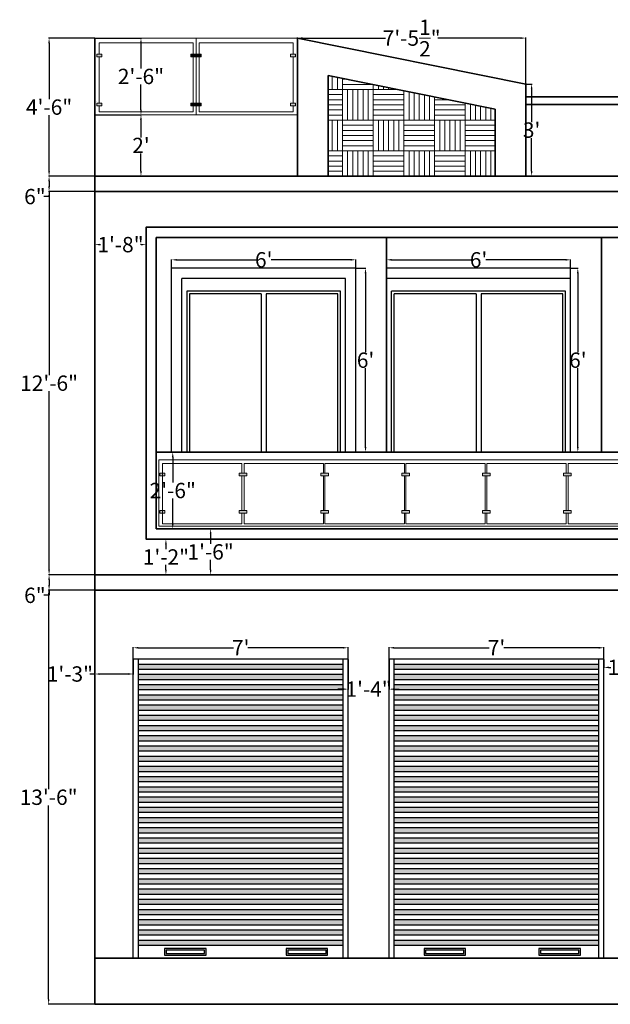
# Model space of a CAD drawing. Units: inches. Extents: x 786 to 1239, y 110 to 563.
# Tile 1 of 3: x 786 to 1017, y 110 to 495. Entities that reach past the tile are written whole.
import ezdxf

# ---------------------------------------------------------------- set-up
doc = ezdxf.new("R2010")
doc.units = ezdxf.units.IN
doc.header["$MEASUREMENT"] = 0
for name, color, linetype, lineweight in [('A-ANNO-DIMS', 2, 'Continuous', 18), ('A-DOOR', 4, 'Continuous', 25), ('A-ELEV', 7, 'Continuous', 35), ('A-ELEV-PATT', 8, 'Continuous', 13), ('A-ELEV-RAIL', 3, 'Continuous', 18), ('A-GLAZ', 4, 'Continuous', 25)]:
    doc.layers.add(name, color=color, linetype=linetype, lineweight=lineweight)
doc.styles.get("Standard").update_dxf_attribs({"font": 'arial.ttf'})
doc.dimstyles.get("Standard").update_dxf_attribs({"dimtxt": 6, "dimasz": 2, "dimexe": 0.18, "dimexo": 0.0625, "dimgap": 0.09, "dimtad": 0, "dimtih": 1, "dimtoh": 1, "dimdec": 1, "dimzin": 0, "dimdsep": 46, "dimlunit": 4, "dimtxsty": 'Standard', "dimcen": 0.09, "dimadec": 0, "dimazin": 0, "dimtfac": 1, "dimtdec": 1, "dimtofl": 0, "dimtmove": 0, "dimatfit": 3, "dimfxl": 1, "dimtolj": 1, "dimtzin": 0, "dimarcsym": 0})

# ---------------------------------------------------------------- blocks, each defined once
blk = doc.blocks.new('*D7')
at = {"layer": 'A-ANNO-DIMS', "color": 0, "lineweight": -2, "transparency": 16777216}
for p, q in [((1035.19, 272.05), (1035.19, 241.73)), ((1014.19, 245.05), (1014.19, 241.73)), ((1016.19, 241.91), (1016.91, 241.91)), ((1033.19, 241.91), (1032.48, 241.91))]:
    blk.add_line(p, q, dxfattribs=at)
at = {"layer": 'A-ANNO-DIMS', "color": 0, "transparency": 16777216}
for points in [[(1016.19, 242.24), (1016.19, 241.58), (1014.19, 241.91)], [(1033.19, 242.24), (1033.19, 241.58), (1035.19, 241.91)]]:
    blk.add_solid(points, dxfattribs=at)
at = {"layer": 'Defpoints', "color": 0, "transparency": 16777216}
for p in [(1035.19, 272.11), (1014.19, 245.11), (1035.19, 241.91)]:
    blk.add_point(p, dxfattribs=at)
at = {"layer": 'A-ANNO-DIMS', "color": 0, "transparency": 16777216, "insert": (1024.69, 241.91), "char_height": 6, "attachment_point": 5}
blk.add_mtext('\\A1;1\'-9"', dxfattribs=at)
blk = doc.blocks.new('*D8')
at = {"layer": 'A-ANNO-DIMS', "color": 0, "lineweight": -2, "transparency": 16777216}
for p, q in [((815.19, 272.05), (815.19, 239.15)), ((830.19, 245.05), (830.19, 239.15)), ((815.19, 239.33), (813.19, 239.33)), ((828.19, 239.33), (817.19, 239.33))]:
    blk.add_line(p, q, dxfattribs=at)
at = {"layer": 'A-ANNO-DIMS', "color": 0, "transparency": 16777216}
for points in [[(817.19, 239.66), (817.19, 238.99), (815.19, 239.33)], [(828.19, 239.66), (828.19, 238.99), (830.19, 239.33)]]:
    blk.add_solid(points, dxfattribs=at)
at = {"layer": 'Defpoints', "color": 0, "transparency": 16777216}
for p in [(815.19, 272.11), (830.19, 245.11), (815.19, 239.33)]:
    blk.add_point(p, dxfattribs=at)
at = {"layer": 'A-ANNO-DIMS', "color": 0, "transparency": 16777216, "insert": (805.41, 239.33), "char_height": 6, "attachment_point": 5}
blk.add_mtext('\\A1;1\'-3"', dxfattribs=at)
blk = doc.blocks.new('*D12')
at = {"layer": 'A-ANNO-DIMS', "color": 0, "lineweight": -2, "transparency": 16777216}
for p, q in [((815.19, 428.05), (815.19, 407.13)), ((835.19, 410.05), (835.19, 407.13)), ((817.19, 407.31), (817.41, 407.31)), ((833.19, 407.31), (832.98, 407.31))]:
    blk.add_line(p, q, dxfattribs=at)
at = {"layer": 'A-ANNO-DIMS', "color": 0, "transparency": 16777216}
for points in [[(817.19, 407.64), (817.19, 406.98), (815.19, 407.31)], [(833.19, 407.64), (833.19, 406.98), (835.19, 407.31)]]:
    blk.add_solid(points, dxfattribs=at)
at = {"layer": 'Defpoints', "color": 0, "transparency": 16777216}
for p in [(815.19, 428.11), (835.19, 410.11), (835.19, 407.31)]:
    blk.add_point(p, dxfattribs=at)
at = {"layer": 'A-ANNO-DIMS', "color": 0, "transparency": 16777216, "insert": (825.19, 407.31), "char_height": 6, "attachment_point": 5}
blk.add_mtext('\\A1;1\'-8"', dxfattribs=at)
blk = doc.blocks.new('*D13')
at = {"layer": 'A-ANNO-DIMS', "color": 0, "lineweight": -2, "transparency": 16777216}
for p, q in [((839.26, 326.11), (845.81, 326.11)), ((845.63, 324.11), (845.63, 314.26)), ((845.63, 298.11), (845.63, 307.96)), ((839.26, 296.11), (845.81, 296.11))]:
    blk.add_line(p, q, dxfattribs=at)
at = {"layer": 'A-ANNO-DIMS', "color": 0, "transparency": 16777216}
for points in [[(845.3, 324.11), (845.97, 324.11), (845.63, 326.11)], [(845.3, 298.11), (845.97, 298.11), (845.63, 296.11)]]:
    blk.add_solid(points, dxfattribs=at)
at = {"layer": 'Defpoints', "color": 0, "transparency": 16777216}
for p in [(839.19, 326.11), (839.19, 296.11), (845.63, 296.11)]:
    blk.add_point(p, dxfattribs=at)
at = {"layer": 'A-ANNO-DIMS', "color": 0, "transparency": 16777216, "insert": (845.63, 311.11), "char_height": 6, "attachment_point": 5}
blk.add_mtext('\\A1;2\'-6"', dxfattribs=at)
blk = doc.blocks.new('*D24')
at = {"layer": 'A-ANNO-DIMS', "color": 0, "lineweight": -2, "transparency": 16777216}
for p, q in [((835.26, 292.11), (843.14, 292.11)), ((842.96, 290.11), (842.96, 288.21)), ((842.96, 280.11), (842.96, 282.01)), ((815.26, 278.11), (843.14, 278.11))]:
    blk.add_line(p, q, dxfattribs=at)
at = {"layer": 'A-ANNO-DIMS', "color": 0, "transparency": 16777216}
for points in [[(842.63, 290.11), (843.29, 290.11), (842.96, 292.11)], [(842.63, 280.11), (843.29, 280.11), (842.96, 278.11)]]:
    blk.add_solid(points, dxfattribs=at)
at = {"layer": 'Defpoints', "color": 0, "transparency": 16777216}
for p in [(835.19, 292.11), (842.96, 292.11), (815.19, 278.11)]:
    blk.add_point(p, dxfattribs=at)
at = {"layer": 'A-ANNO-DIMS', "color": 0, "transparency": 16777216, "insert": (842.96, 285.11), "char_height": 6, "attachment_point": 5}
blk.add_mtext('\\A1;1\'-2"', dxfattribs=at)
blk = doc.blocks.new('*D25')
at = {"layer": 'A-ANNO-DIMS', "color": 0, "lineweight": -2, "transparency": 16777216}
for p, q in [((839.26, 296.11), (860.61, 296.11)), ((860.43, 294.11), (860.43, 290.26)), ((860.43, 280.11), (860.43, 283.96)), ((815.26, 278.11), (860.61, 278.11))]:
    blk.add_line(p, q, dxfattribs=at)
at = {"layer": 'A-ANNO-DIMS', "color": 0, "transparency": 16777216}
for points in [[(860.1, 294.11), (860.77, 294.11), (860.43, 296.11)], [(860.1, 280.11), (860.77, 280.11), (860.43, 278.11)]]:
    blk.add_solid(points, dxfattribs=at)
at = {"layer": 'Defpoints', "color": 0, "transparency": 16777216}
for p in [(839.19, 296.11), (860.43, 296.11), (815.19, 278.11)]:
    blk.add_point(p, dxfattribs=at)
at = {"layer": 'A-ANNO-DIMS', "color": 0, "transparency": 16777216, "insert": (860.43, 287.11), "char_height": 6, "attachment_point": 5}
blk.add_mtext('\\A1;1\'-6"', dxfattribs=at)
blk = doc.blocks.new('*D26')
at = {"layer": 'A-ANNO-DIMS', "color": 0, "lineweight": -2, "transparency": 16777216}
for p, q in [((894.39, 488.17), (894.39, 488.29)), ((896.39, 488.11), (928.8, 488.11)), ((981.67, 488.11), (949.26, 488.11)), ((983.67, 470.19), (983.67, 488.29))]:
    blk.add_line(p, q, dxfattribs=at)
at = {"layer": 'A-ANNO-DIMS', "color": 0, "transparency": 16777216}
for points in [[(896.39, 488.44), (896.39, 487.78), (894.39, 488.11)], [(981.67, 488.44), (981.67, 487.78), (983.67, 488.11)]]:
    blk.add_solid(points, dxfattribs=at)
at = {"layer": 'Defpoints', "color": 0, "transparency": 16777216}
for p in [(894.39, 488.11), (894.39, 488.11), (983.67, 470.13)]:
    blk.add_point(p, dxfattribs=at)
at = {"layer": 'A-ANNO-DIMS', "color": 0, "transparency": 16777216, "insert": (939.03, 488.11), "char_height": 6, "attachment_point": 5}
blk.add_mtext('\\A1;7\'-5{\\H1x;\\S1/2;}"', dxfattribs=at)
blk = doc.blocks.new('*D27')
at = {"layer": 'A-ANNO-DIMS', "color": 0, "lineweight": -2, "transparency": 16777216}
for p, q in [((983.73, 470.13), (986.11, 470.13)), ((985.93, 468.13), (985.93, 455.27)), ((985.93, 436.11), (985.93, 448.96)), ((983.73, 434.11), (986.11, 434.11))]:
    blk.add_line(p, q, dxfattribs=at)
at = {"layer": 'A-ANNO-DIMS', "color": 0, "transparency": 16777216}
for points in [[(985.6, 468.13), (986.27, 468.13), (985.93, 470.13)], [(985.6, 436.11), (986.27, 436.11), (985.93, 434.11)]]:
    blk.add_solid(points, dxfattribs=at)
at = {"layer": 'Defpoints', "color": 0, "transparency": 16777216}
for p in [(983.67, 470.13), (985.93, 470.13), (983.67, 434.11)]:
    blk.add_point(p, dxfattribs=at)
at = {"layer": 'A-ANNO-DIMS', "color": 0, "transparency": 16777216, "insert": (985.93, 452.12), "char_height": 6, "attachment_point": 5}
blk.add_mtext("\\A1;3'", dxfattribs=at)
blk = doc.blocks.new('*D28')
at = {"layer": 'A-ANNO-DIMS', "color": 0, "lineweight": -2, "transparency": 16777216}
for p, q in [((815.26, 488.11), (833.38, 488.11)), ((833.2, 486.11), (833.2, 476.26)), ((833.2, 460.11), (833.2, 469.96)), ((815.26, 458.11), (833.38, 458.11))]:
    blk.add_line(p, q, dxfattribs=at)
at = {"layer": 'A-ANNO-DIMS', "color": 0, "transparency": 16777216}
for points in [[(832.86, 486.11), (833.53, 486.11), (833.2, 488.11)], [(832.86, 460.11), (833.53, 460.11), (833.2, 458.11)]]:
    blk.add_solid(points, dxfattribs=at)
at = {"layer": 'Defpoints', "color": 0, "transparency": 16777216}
for p in [(815.19, 488.11), (815.19, 458.11), (833.2, 458.11)]:
    blk.add_point(p, dxfattribs=at)
at = {"layer": 'A-ANNO-DIMS', "color": 0, "transparency": 16777216, "insert": (833.2, 473.11), "char_height": 6, "attachment_point": 5}
blk.add_mtext('\\A1;2\'-6"', dxfattribs=at)
blk = doc.blocks.new('*D29')
at = {"layer": 'A-ANNO-DIMS', "color": 0, "lineweight": -2, "transparency": 16777216}
for p, q in [((815.26, 458.11), (833.38, 458.11)), ((833.2, 456.11), (833.2, 449.21)), ((833.2, 436.11), (833.2, 443.01)), ((815.26, 434.11), (833.38, 434.11))]:
    blk.add_line(p, q, dxfattribs=at)
at = {"layer": 'A-ANNO-DIMS', "color": 0, "transparency": 16777216}
for points in [[(832.86, 456.11), (833.53, 456.11), (833.2, 458.11)], [(832.86, 436.11), (833.53, 436.11), (833.2, 434.11)]]:
    blk.add_solid(points, dxfattribs=at)
at = {"layer": 'Defpoints', "color": 0, "transparency": 16777216}
for p in [(815.19, 458.11), (815.19, 434.11), (833.2, 434.11)]:
    blk.add_point(p, dxfattribs=at)
at = {"layer": 'A-ANNO-DIMS', "color": 0, "transparency": 16777216, "insert": (833.2, 446.11), "char_height": 6, "attachment_point": 5}
blk.add_mtext("\\A1;2'", dxfattribs=at)
blk = doc.blocks.new('*D30')
at = {"layer": 'A-ANNO-DIMS', "color": 0, "lineweight": -2, "transparency": 16777216}
for p, q in [((830.19, 245.17), (830.19, 249.77)), ((832.19, 249.59), (869.37, 249.59)), ((912.19, 249.59), (875.02, 249.59)), ((914.19, 245.17), (914.19, 249.77))]:
    blk.add_line(p, q, dxfattribs=at)
at = {"layer": 'A-ANNO-DIMS', "color": 0, "transparency": 16777216}
for points in [[(832.19, 249.92), (832.19, 249.26), (830.19, 249.59)], [(912.19, 249.92), (912.19, 249.26), (914.19, 249.59)]]:
    blk.add_solid(points, dxfattribs=at)
at = {"layer": 'Defpoints', "color": 0, "transparency": 16777216}
for p in [(830.19, 249.59), (830.19, 245.11), (914.19, 245.11)]:
    blk.add_point(p, dxfattribs=at)
at = {"layer": 'A-ANNO-DIMS', "color": 0, "transparency": 16777216, "insert": (872.19, 249.59), "char_height": 6, "attachment_point": 5}
blk.add_mtext("\\A1;7'", dxfattribs=at)
blk = doc.blocks.new('*D31')
at = {"layer": 'A-ANNO-DIMS', "color": 0, "lineweight": -2, "transparency": 16777216}
for p, q in [((930.19, 245.17), (930.19, 249.77)), ((932.19, 249.59), (969.37, 249.59)), ((1012.19, 249.59), (975.02, 249.59)), ((1014.19, 245.17), (1014.19, 249.77))]:
    blk.add_line(p, q, dxfattribs=at)
at = {"layer": 'A-ANNO-DIMS', "color": 0, "transparency": 16777216}
for points in [[(932.19, 249.92), (932.19, 249.26), (930.19, 249.59)], [(1012.19, 249.92), (1012.19, 249.26), (1014.19, 249.59)]]:
    blk.add_solid(points, dxfattribs=at)
at = {"layer": 'Defpoints', "color": 0, "transparency": 16777216}
for p in [(930.19, 249.59), (930.19, 245.11), (1014.19, 245.11)]:
    blk.add_point(p, dxfattribs=at)
at = {"layer": 'A-ANNO-DIMS', "color": 0, "transparency": 16777216, "insert": (972.19, 249.59), "char_height": 6, "attachment_point": 5}
blk.add_mtext("\\A1;7'", dxfattribs=at)
blk = doc.blocks.new('*D32')
at = {"layer": 'A-ANNO-DIMS', "color": 0, "lineweight": -2, "transparency": 16777216}
for p, q in [((914.19, 245.05), (914.19, 233.22)), ((930.19, 245.05), (930.19, 233.22)), ((912.19, 233.4), (910.19, 233.4)), ((932.19, 233.4), (934.19, 233.4))]:
    blk.add_line(p, q, dxfattribs=at)
at = {"layer": 'A-ANNO-DIMS', "color": 0, "transparency": 16777216}
for points in [[(912.19, 233.74), (912.19, 233.07), (914.19, 233.4)], [(932.19, 233.74), (932.19, 233.07), (930.19, 233.4)]]:
    blk.add_solid(points, dxfattribs=at)
at = {"layer": 'Defpoints', "color": 0, "transparency": 16777216}
for p in [(914.19, 245.11), (930.19, 245.11), (930.19, 233.4)]:
    blk.add_point(p, dxfattribs=at)
at = {"layer": 'A-ANNO-DIMS', "color": 0, "transparency": 16777216, "insert": (922.19, 233.4), "char_height": 6, "attachment_point": 5}
blk.add_mtext('\\A1;1\'-4"', dxfattribs=at)
blk = doc.blocks.new('*D43')
at = {"layer": 'A-ANNO-DIMS', "color": 0, "lineweight": -2, "transparency": 16777216}
for p, q in [((815.13, 278.11), (797.1, 278.11)), ((797.28, 276.11), (797.28, 274.11)), ((797.28, 270.11), (795.28, 270.11)), ((815.13, 272.11), (797.1, 272.11)), ((797.28, 272.11), (797.28, 270.11))]:
    blk.add_line(p, q, dxfattribs=at)
at = {"layer": 'A-ANNO-DIMS', "color": 0, "transparency": 16777216}
for points in [[(796.95, 276.11), (797.61, 276.11), (797.28, 278.11)], [(796.95, 274.11), (797.61, 274.11), (797.28, 272.11)]]:
    blk.add_solid(points, dxfattribs=at)
at = {"layer": 'Defpoints', "color": 0, "transparency": 16777216}
for p in [(815.19, 278.11), (797.28, 272.11), (815.19, 272.11)]:
    blk.add_point(p, dxfattribs=at)
at = {"layer": 'A-ANNO-DIMS', "color": 0, "transparency": 16777216, "insert": (791.73, 270.11), "char_height": 6, "attachment_point": 5}
blk.add_mtext('\\A1;6"', dxfattribs=at)
blk = doc.blocks.new('*D44')
at = {"layer": 'A-ANNO-DIMS', "color": 0, "lineweight": -2, "transparency": 16777216}
for p, q in [((815.13, 272.11), (796.92, 272.11)), ((797.1, 270.11), (797.1, 194.26)), ((797.1, 112.11), (797.1, 187.95)), ((815.13, 110.11), (796.92, 110.11))]:
    blk.add_line(p, q, dxfattribs=at)
at = {"layer": 'A-ANNO-DIMS', "color": 0, "transparency": 16777216}
for points in [[(796.77, 270.11), (797.43, 270.11), (797.1, 272.11)], [(796.77, 112.11), (797.43, 112.11), (797.1, 110.11)]]:
    blk.add_solid(points, dxfattribs=at)
at = {"layer": 'Defpoints', "color": 0, "transparency": 16777216}
for p in [(815.19, 272.11), (797.1, 110.11), (815.19, 110.11)]:
    blk.add_point(p, dxfattribs=at)
at = {"layer": 'A-ANNO-DIMS', "color": 0, "transparency": 16777216, "insert": (797.1, 191.11), "char_height": 6, "attachment_point": 5}
blk.add_mtext('\\A1;13\'-6"', dxfattribs=at)
blk = doc.blocks.new('*D45')
at = {"layer": 'A-ANNO-DIMS', "color": 0, "lineweight": -2, "transparency": 16777216}
for p, q in [((815.13, 428.11), (797.1, 428.11)), ((797.28, 426.11), (797.28, 356.26)), ((797.28, 280.11), (797.28, 349.96)), ((815.13, 278.11), (797.1, 278.11))]:
    blk.add_line(p, q, dxfattribs=at)
at = {"layer": 'A-ANNO-DIMS', "color": 0, "transparency": 16777216}
for points in [[(796.95, 426.11), (797.61, 426.11), (797.28, 428.11)], [(796.95, 280.11), (797.61, 280.11), (797.28, 278.11)]]:
    blk.add_solid(points, dxfattribs=at)
at = {"layer": 'Defpoints', "color": 0, "transparency": 16777216}
for p in [(797.28, 428.11), (815.19, 428.11), (815.19, 278.11)]:
    blk.add_point(p, dxfattribs=at)
at = {"layer": 'A-ANNO-DIMS', "color": 0, "transparency": 16777216, "insert": (797.28, 353.11), "char_height": 6, "attachment_point": 5}
blk.add_mtext('\\A1;12\'-6"', dxfattribs=at)
blk = doc.blocks.new('*D46')
at = {"layer": 'A-ANNO-DIMS', "color": 0, "lineweight": -2, "transparency": 16777216}
for p, q in [((815.13, 434.11), (797.1, 434.11)), ((797.28, 432.11), (797.28, 430.11)), ((815.13, 428.11), (797.1, 428.11)), ((797.28, 428.11), (797.28, 426.11)), ((797.28, 426.11), (795.28, 426.11))]:
    blk.add_line(p, q, dxfattribs=at)
at = {"layer": 'A-ANNO-DIMS', "color": 0, "transparency": 16777216}
for points in [[(796.95, 432.11), (797.61, 432.11), (797.28, 434.11)], [(796.95, 430.11), (797.61, 430.11), (797.28, 428.11)]]:
    blk.add_solid(points, dxfattribs=at)
at = {"layer": 'Defpoints', "color": 0, "transparency": 16777216}
for p in [(815.19, 434.11), (797.28, 428.11), (815.19, 428.11)]:
    blk.add_point(p, dxfattribs=at)
at = {"layer": 'A-ANNO-DIMS', "color": 0, "transparency": 16777216, "insert": (791.73, 426.11), "char_height": 6, "attachment_point": 5}
blk.add_mtext('\\A1;6"', dxfattribs=at)
blk = doc.blocks.new('*D47')
at = {"layer": 'A-ANNO-DIMS', "color": 0, "lineweight": -2, "transparency": 16777216}
for p, q in [((815.13, 488.11), (797.1, 488.11)), ((797.28, 486.11), (797.28, 464.26)), ((797.28, 436.11), (797.28, 457.96)), ((815.13, 434.11), (797.1, 434.11))]:
    blk.add_line(p, q, dxfattribs=at)
at = {"layer": 'A-ANNO-DIMS', "color": 0, "transparency": 16777216}
for points in [[(796.95, 486.11), (797.61, 486.11), (797.28, 488.11)], [(796.95, 436.11), (797.61, 436.11), (797.28, 434.11)]]:
    blk.add_solid(points, dxfattribs=at)
at = {"layer": 'Defpoints', "color": 0, "transparency": 16777216}
for p in [(797.28, 488.11), (815.19, 488.11), (815.19, 434.11)]:
    blk.add_point(p, dxfattribs=at)
at = {"layer": 'A-ANNO-DIMS', "color": 0, "transparency": 16777216, "insert": (797.28, 461.11), "char_height": 6, "attachment_point": 5}
blk.add_mtext('\\A1;4\'-6"', dxfattribs=at)
blk = doc.blocks.new('*D51')
at = {"layer": 'A-ANNO-DIMS', "color": 0, "lineweight": -2, "transparency": 16777216}
for p, q in [((929.19, 398.17), (929.19, 401.55)), ((931.19, 401.37), (962.33, 401.37)), ((999.19, 401.37), (968.06, 401.37)), ((1001.19, 398.17), (1001.19, 401.55))]:
    blk.add_line(p, q, dxfattribs=at)
at = {"layer": 'A-ANNO-DIMS', "color": 0, "transparency": 16777216}
for points in [[(931.19, 401.7), (931.19, 401.03), (929.19, 401.37)], [(999.19, 401.7), (999.19, 401.03), (1001.19, 401.37)]]:
    blk.add_solid(points, dxfattribs=at)
at = {"layer": 'Defpoints', "color": 0, "transparency": 16777216}
for p in [(929.19, 401.37), (929.19, 398.11), (1001.19, 398.11)]:
    blk.add_point(p, dxfattribs=at)
at = {"layer": 'A-ANNO-DIMS', "color": 0, "transparency": 16777216, "insert": (965.19, 401.37), "char_height": 6, "attachment_point": 5}
blk.add_mtext("\\A1;6'", dxfattribs=at)
blk = doc.blocks.new('*D52')
at = {"layer": 'A-ANNO-DIMS', "color": 0, "lineweight": -2, "transparency": 16777216}
for p, q in [((845.19, 398.17), (845.19, 401.55)), ((847.19, 401.37), (878.33, 401.37)), ((915.19, 401.37), (884.06, 401.37)), ((917.19, 398.17), (917.19, 401.55))]:
    blk.add_line(p, q, dxfattribs=at)
at = {"layer": 'A-ANNO-DIMS', "color": 0, "transparency": 16777216}
for points in [[(847.19, 401.7), (847.19, 401.03), (845.19, 401.37)], [(915.19, 401.7), (915.19, 401.03), (917.19, 401.37)]]:
    blk.add_solid(points, dxfattribs=at)
at = {"layer": 'Defpoints', "color": 0, "transparency": 16777216}
for p in [(845.19, 401.37), (845.19, 398.11), (917.19, 398.11)]:
    blk.add_point(p, dxfattribs=at)
at = {"layer": 'A-ANNO-DIMS', "color": 0, "transparency": 16777216, "insert": (881.19, 401.37), "char_height": 6, "attachment_point": 5}
blk.add_mtext("\\A1;6'", dxfattribs=at)
blk = doc.blocks.new('*D53')
at = {"layer": 'A-ANNO-DIMS', "color": 0, "lineweight": -2, "transparency": 16777216}
for p, q in [((917.26, 398.11), (921.18, 398.11)), ((921, 396.11), (921, 365.26)), ((921, 328.11), (921, 358.96)), ((917.26, 326.11), (921.18, 326.11))]:
    blk.add_line(p, q, dxfattribs=at)
at = {"layer": 'A-ANNO-DIMS', "color": 0, "transparency": 16777216}
for points in [[(920.66, 396.11), (921.33, 396.11), (921, 398.11)], [(920.66, 328.11), (921.33, 328.11), (921, 326.11)]]:
    blk.add_solid(points, dxfattribs=at)
at = {"layer": 'Defpoints', "color": 0, "transparency": 16777216}
for p in [(917.19, 398.11), (921, 398.11), (917.19, 326.11)]:
    blk.add_point(p, dxfattribs=at)
at = {"layer": 'A-ANNO-DIMS', "color": 0, "transparency": 16777216, "insert": (921, 362.11), "char_height": 6, "attachment_point": 5}
blk.add_mtext("\\A1;6'", dxfattribs=at)
blk = doc.blocks.new('*D54')
at = {"layer": 'A-ANNO-DIMS', "color": 0, "lineweight": -2, "transparency": 16777216}
for p, q in [((1001.26, 398.11), (1004.18, 398.11)), ((1004, 396.11), (1004, 365.26)), ((1004, 328.11), (1004, 358.96)), ((1001.26, 326.11), (1004.18, 326.11))]:
    blk.add_line(p, q, dxfattribs=at)
at = {"layer": 'A-ANNO-DIMS', "color": 0, "transparency": 16777216}
for points in [[(1003.66, 396.11), (1004.33, 396.11), (1004, 398.11)], [(1003.66, 328.11), (1004.33, 328.11), (1004, 326.11)]]:
    blk.add_solid(points, dxfattribs=at)
at = {"layer": 'Defpoints', "color": 0, "transparency": 16777216}
for p in [(1001.19, 398.11), (1004, 398.11), (1001.19, 326.11)]:
    blk.add_point(p, dxfattribs=at)
at = {"layer": 'A-ANNO-DIMS', "color": 0, "transparency": 16777216, "insert": (1004, 362.11), "char_height": 6, "attachment_point": 5}
blk.add_mtext("\\A1;6'", dxfattribs=at)
blk = doc.blocks.new('GLASS-CLAMP-A')
for p, q in [((0, 1), (3, 1)), ((0, 1), (0, 0)), ((3, 0), (3, 1)), ((3, 0), (0, 0))]:
    blk.add_line(p, q)
blk = doc.blocks.new('GLASS-CLAMP-B')
for p, q in [((0, 1), (2, 1)), ((0, 0), (0, 1)), ((2, 0), (2, 1)), ((0, 0), (2, 0))]:
    blk.add_line(p, q)
blk = doc.blocks.new('GLASS-CLAMP-C')
for p, q in [((0, 1), (4, 1)), ((0, 1), (0, 0)), ((4, 1), (4, 0)), ((0, 0), (4, 0))]:
    blk.add_line(p, q)
blk = doc.blocks.new('ROLLING-SHUTTER-FRAME')
for p, q in [((0, 0), (0, 117)), ((84, 117), (0, 117)), ((84, 0), (84, 117))]:
    blk.add_line(p, q)

msp = doc.modelspace()

# ---------------------------------------------------------------- hatches: boundary and pattern name
at = {"layer": 'A-ELEV-PATT'}
h = msp.add_hatch(color=256, dxfattribs=at)
h.dxf.hatch_style = 1
h.paths.add_polyline_path([(817.91, 481.76), (815.91, 481.76), (815.91, 480.76), (817.91, 480.76)])
h.paths.add_polyline_path([(817.91, 462.63), (815.91, 462.63), (815.91, 461.64), (817.91, 461.64)])
h.paths.add_polyline_path([(893.66, 481.76), (891.66, 481.76), (891.66, 480.76), (893.66, 480.76)])
h.paths.add_polyline_path([(893.66, 462.63), (891.66, 462.63), (891.66, 461.64), (893.66, 461.64)])
h = msp.add_hatch(color=256, dxfattribs=at)
h.dxf.hatch_style = 1
h.paths.add_polyline_path([(854.79, 481.76), (853.67, 481.76), (853.67, 480.76), (854.79, 480.76)])
h.paths.add_polyline_path([(853.67, 481.76), (852.69, 481.76), (852.69, 480.76), (853.67, 480.76)])
h.paths.add_polyline_path([(855.9, 481.76), (854.79, 481.76), (854.79, 480.76), (855.9, 480.76)])
h.paths.add_polyline_path([(856.69, 481.76), (855.9, 481.76), (855.9, 480.76), (856.69, 480.76)])
h = msp.add_hatch(dxfattribs=at)
h.set_pattern_fill('AR-PARQ1', color=256)
h.paths.add_polyline_path([(971.67, 460.3), (906.39, 473.45), (906.39, 434.11), (971.67, 434.11)])
h = msp.add_hatch(color=256, dxfattribs=at)
h.dxf.hatch_style = 1
h.paths.add_polyline_path([(854.79, 462.64), (853.67, 462.64), (853.67, 461.64), (854.79, 461.64)])
h.paths.add_polyline_path([(853.67, 462.64), (852.69, 462.64), (852.69, 461.64), (853.67, 461.64)])
h.paths.add_polyline_path([(855.9, 462.64), (854.79, 462.64), (854.79, 461.64), (855.9, 461.64)])
h.paths.add_polyline_path([(856.69, 462.64), (855.9, 462.64), (855.9, 461.64), (856.69, 461.64)])
h = msp.add_hatch(color=256, dxfattribs=at)
h.dxf.hatch_style = 1
h.paths.add_polyline_path([(842.59, 317.86), (841.59, 317.86), (841.59, 316.86), (842.59, 316.86)])
h.paths.add_polyline_path([(841.59, 317.86), (840.59, 317.86), (840.59, 316.86), (841.59, 316.86)])
h.paths.add_polyline_path([(842.59, 303.29), (841.59, 303.29), (841.59, 302.31), (842.59, 302.31)])
h.paths.add_polyline_path([(841.59, 303.29), (840.59, 303.29), (840.59, 302.31), (841.59, 302.31)])
h.paths.add_polyline_path([(1064.36, 317.86), (1063.36, 317.86), (1063.36, 316.86), (1064.36, 316.86)])
h.paths.add_polyline_path([(1063.36, 317.86), (1062.36, 317.86), (1062.36, 316.86), (1063.36, 316.86)])
h.paths.add_polyline_path([(1064.36, 303.29), (1063.36, 303.29), (1063.36, 302.31), (1064.36, 302.31)])
h.paths.add_polyline_path([(1063.36, 303.29), (1062.36, 303.29), (1062.36, 302.31), (1063.36, 302.31)])
h = msp.add_hatch(color=256, dxfattribs=at)
h.dxf.hatch_style = 1
h.paths.add_polyline_path([(874.65, 317.86), (871.65, 317.86), (871.65, 316.86), (874.65, 316.86)])
h.paths.add_polyline_path([(906.56, 317.86), (903.56, 317.86), (903.56, 316.86), (906.56, 316.86)])
h.paths.add_polyline_path([(938.2, 317.86), (935.2, 317.86), (935.2, 316.86), (938.2, 316.86)])
h.paths.add_polyline_path([(969.78, 317.86), (966.78, 317.86), (966.78, 316.86), (969.78, 316.86)])
h.paths.add_polyline_path([(1001.46, 317.86), (998.46, 317.86), (998.46, 316.86), (1001.46, 316.86)])
h.paths.add_polyline_path([(1033.24, 317.86), (1030.24, 317.86), (1030.24, 316.86), (1033.24, 316.86)])
h.paths.add_polyline_path([(1033.24, 303.31), (1030.24, 303.31), (1030.24, 302.31), (1033.24, 302.31)])
h.paths.add_polyline_path([(1001.46, 303.31), (998.46, 303.31), (998.46, 302.31), (1001.46, 302.31)])
h.paths.add_polyline_path([(969.78, 303.31), (966.78, 303.31), (966.78, 302.31), (969.78, 302.31)])
h.paths.add_polyline_path([(938.2, 303.31), (935.2, 303.31), (935.2, 302.31), (938.2, 302.31)])
h.paths.add_polyline_path([(906.56, 303.31), (903.56, 303.31), (903.56, 302.31), (906.56, 302.31)])
h.paths.add_polyline_path([(874.65, 303.31), (871.65, 303.31), (871.65, 302.31), (874.65, 302.31)])
h = msp.add_hatch(color=256, dxfattribs=at)
h.dxf.hatch_style = 1
h.paths.add_polyline_path([(912.19, 243.11), (832.19, 243.11), (832.19, 241.11), (912.19, 241.11)])
h.paths.add_polyline_path([(912.19, 239.11), (832.19, 239.11), (832.19, 237.11), (912.19, 237.11)])
h.paths.add_polyline_path([(912.19, 235.11), (832.19, 235.11), (832.19, 233.11), (912.19, 233.11)])
h.paths.add_polyline_path([(912.19, 231.11), (832.19, 231.11), (832.19, 229.11), (912.19, 229.11)])
h.paths.add_polyline_path([(912.19, 227.11), (832.19, 227.11), (832.19, 225.11), (912.19, 225.11)])
h.paths.add_polyline_path([(912.19, 223.11), (832.19, 223.11), (832.19, 221.11), (912.19, 221.11)])
h.paths.add_polyline_path([(912.19, 219.11), (832.19, 219.11), (832.19, 217.11), (912.19, 217.11)])
h.paths.add_polyline_path([(912.19, 215.11), (832.19, 215.11), (832.19, 213.11), (912.19, 213.11)])
h.paths.add_polyline_path([(912.19, 211.11), (832.19, 211.11), (832.19, 209.11), (912.19, 209.11)])
h.paths.add_polyline_path([(912.19, 207.11), (832.19, 207.11), (832.19, 205.11), (912.19, 205.11)])
h.paths.add_polyline_path([(912.19, 203.11), (832.19, 203.11), (832.19, 201.11), (912.19, 201.11)])
h.paths.add_polyline_path([(912.19, 199.11), (832.19, 199.11), (832.19, 197.11), (912.19, 197.11)])
h.paths.add_polyline_path([(912.19, 195.11), (832.19, 195.11), (832.19, 193.11), (912.19, 193.11)])
h.paths.add_polyline_path([(912.19, 191.11), (832.19, 191.11), (832.19, 189.11), (912.19, 189.11)])
h.paths.add_polyline_path([(912.19, 187.11), (832.19, 187.11), (832.19, 185.11), (912.19, 185.11)])
h.paths.add_polyline_path([(912.19, 183.11), (832.19, 183.11), (832.19, 181.11), (912.19, 181.11)])
h.paths.add_polyline_path([(912.19, 179.11), (832.19, 179.11), (832.19, 177.11), (912.19, 177.11)])
h.paths.add_polyline_path([(912.19, 175.11), (832.19, 175.11), (832.19, 173.11), (912.19, 173.11)])
h.paths.add_polyline_path([(912.19, 171.11), (832.19, 171.11), (832.19, 169.11), (912.19, 169.11)])
h.paths.add_polyline_path([(912.19, 167.11), (832.19, 167.11), (832.19, 165.11), (912.19, 165.11)])
h.paths.add_polyline_path([(912.19, 163.11), (832.19, 163.11), (832.19, 161.11), (912.19, 161.11)])
h.paths.add_polyline_path([(912.19, 159.11), (832.19, 159.11), (832.19, 157.11), (912.19, 157.11)])
h.paths.add_polyline_path([(912.19, 155.11), (832.19, 155.11), (832.19, 153.11), (912.19, 153.11)])
h.paths.add_polyline_path([(912.19, 151.11), (832.19, 151.11), (832.19, 149.11), (912.19, 149.11)])
h.paths.add_polyline_path([(912.19, 147.11), (832.19, 147.11), (832.19, 145.11), (912.19, 145.11)])
h.paths.add_polyline_path([(912.19, 143.11), (832.19, 143.11), (832.19, 141.11), (912.19, 141.11)])
h.paths.add_polyline_path([(912.19, 139.11), (832.19, 139.11), (832.19, 137.11), (912.19, 137.11)])
h.paths.add_polyline_path([(912.19, 135.11), (832.19, 135.11), (832.19, 133.11), (912.19, 133.11)])
h = msp.add_hatch(color=256, dxfattribs=at)
h.dxf.hatch_style = 1
h.paths.add_polyline_path([(1012.19, 243.11), (932.19, 243.11), (932.19, 241.11), (1012.19, 241.11)])
h.paths.add_polyline_path([(1012.19, 239.11), (932.19, 239.11), (932.19, 237.11), (1012.19, 237.11)])
h.paths.add_polyline_path([(1012.19, 235.11), (932.19, 235.11), (932.19, 233.11), (1012.19, 233.11)])
h.paths.add_polyline_path([(1012.19, 231.11), (932.19, 231.11), (932.19, 229.11), (1012.19, 229.11)])
h.paths.add_polyline_path([(1012.19, 227.11), (932.19, 227.11), (932.19, 225.11), (1012.19, 225.11)])
h.paths.add_polyline_path([(1012.19, 223.11), (932.19, 223.11), (932.19, 221.11), (1012.19, 221.11)])
h.paths.add_polyline_path([(1012.19, 219.11), (932.19, 219.11), (932.19, 217.11), (1012.19, 217.11)])
h.paths.add_polyline_path([(1012.19, 215.11), (932.19, 215.11), (932.19, 213.11), (1012.19, 213.11)])
h.paths.add_polyline_path([(1012.19, 211.11), (932.19, 211.11), (932.19, 209.11), (1012.19, 209.11)])
h.paths.add_polyline_path([(1012.19, 207.11), (932.19, 207.11), (932.19, 205.11), (1012.19, 205.11)])
h.paths.add_polyline_path([(1012.19, 203.11), (932.19, 203.11), (932.19, 201.11), (1012.19, 201.11)])
h.paths.add_polyline_path([(1012.19, 199.11), (932.19, 199.11), (932.19, 197.11), (1012.19, 197.11)])
h.paths.add_polyline_path([(1012.19, 195.11), (932.19, 195.11), (932.19, 193.11), (1012.19, 193.11)])
h.paths.add_polyline_path([(1012.19, 191.11), (932.19, 191.11), (932.19, 189.11), (1012.19, 189.11)])
h.paths.add_polyline_path([(1012.19, 187.11), (932.19, 187.11), (932.19, 185.11), (1012.19, 185.11)])
h.paths.add_polyline_path([(1012.19, 183.11), (932.19, 183.11), (932.19, 181.11), (1012.19, 181.11)])
h.paths.add_polyline_path([(1012.19, 179.11), (932.19, 179.11), (932.19, 177.11), (1012.19, 177.11)])
h.paths.add_polyline_path([(1012.19, 175.11), (932.19, 175.11), (932.19, 173.11), (1012.19, 173.11)])
h.paths.add_polyline_path([(1012.19, 171.11), (932.19, 171.11), (932.19, 169.11), (1012.19, 169.11)])
h.paths.add_polyline_path([(1012.19, 167.11), (932.19, 167.11), (932.19, 165.11), (1012.19, 165.11)])
h.paths.add_polyline_path([(1012.19, 163.11), (932.19, 163.11), (932.19, 161.11), (1012.19, 161.11)])
h.paths.add_polyline_path([(1012.19, 159.11), (932.19, 159.11), (932.19, 157.11), (1012.19, 157.11)])
h.paths.add_polyline_path([(1012.19, 155.11), (932.19, 155.11), (932.19, 153.11), (1012.19, 153.11)])
h.paths.add_polyline_path([(1012.19, 151.11), (932.19, 151.11), (932.19, 149.11), (1012.19, 149.11)])
h.paths.add_polyline_path([(1012.19, 147.11), (932.19, 147.11), (932.19, 145.11), (1012.19, 145.11)])
h.paths.add_polyline_path([(1012.19, 143.11), (932.19, 143.11), (932.19, 141.11), (1012.19, 141.11)])
h.paths.add_polyline_path([(1012.19, 139.11), (932.19, 139.11), (932.19, 137.11), (1012.19, 137.11)])
h.paths.add_polyline_path([(1012.19, 135.11), (932.19, 135.11), (932.19, 133.11), (1012.19, 133.11)])
h = msp.add_hatch(color=256, dxfattribs=at)
h.dxf.hatch_style = 1
h.paths.add_polyline_path([(1005.02, 131.91), (988.77, 131.91), (988.77, 129.39), (1005.02, 129.39)])
h.paths.add_polyline_path([(1004.38, 130.02), (989.41, 130.02), (989.41, 131.28), (1004.38, 131.28)], flags=16)
h.paths.add_polyline_path([(960.11, 131.91), (943.86, 131.91), (943.86, 129.39), (960.11, 129.39)])
h.paths.add_polyline_path([(959.47, 130.02), (944.49, 130.02), (944.49, 131.28), (959.47, 131.28)], flags=16)
h.paths.add_polyline_path([(906.18, 131.91), (889.93, 131.91), (889.93, 129.39), (906.18, 129.39)])
h.paths.add_polyline_path([(905.55, 130.02), (890.57, 130.02), (890.57, 131.28), (905.55, 131.28)], flags=16)
h.paths.add_polyline_path([(858.63, 131.91), (842.38, 131.91), (842.38, 129.39), (858.63, 129.39)])
h.paths.add_polyline_path([(857.99, 130.02), (843.02, 130.02), (843.02, 131.28), (857.99, 131.28)], flags=16)

# ---------------------------------------------------------------- linework, layer by layer
at = {"layer": 'A-DOOR'}
for p, q in [((832.19, 128.11), (832.19, 245.11)), ((912.19, 243.11), (832.19, 243.11)), ((912.19, 128.11), (912.19, 245.11)), ((932.19, 128.11), (932.19, 245.11)), ((1012.19, 243.11), (932.19, 243.11)), ((1012.19, 128.11), (1012.19, 245.11)), ((912.19, 241.11), (832.19, 241.11)), ((912.19, 239.11), (832.19, 239.11)), ((1012.19, 241.11), (932.19, 241.11)), ((1012.19, 239.11), (932.19, 239.11)), ((912.19, 237.11), (832.19, 237.11)), ((912.19, 235.11), (832.19, 235.11)), ((1012.19, 237.11), (932.19, 237.11)), ((1012.19, 235.11), (932.19, 235.11)), ((912.19, 233.11), (832.19, 233.11)), ((1012.19, 233.11), (932.19, 233.11)), ((912.19, 231.11), (832.19, 231.11)), ((912.19, 229.11), (832.19, 229.11)), ((1012.19, 231.11), (932.19, 231.11)), ((1012.19, 229.11), (932.19, 229.11)), ((912.19, 227.11), (832.19, 227.11)), ((912.19, 225.11), (832.19, 225.11)), ((1012.19, 227.11), (932.19, 227.11)), ((1012.19, 225.11), (932.19, 225.11)), ((912.19, 223.11), (832.19, 223.11)), ((912.19, 221.11), (832.19, 221.11)), ((1012.19, 223.11), (932.19, 223.11)), ((1012.19, 221.11), (932.19, 221.11)), ((912.19, 219.11), (832.19, 219.11)), ((912.19, 217.11), (832.19, 217.11)), ((1012.19, 219.11), (932.19, 219.11)), ((1012.19, 217.11), (932.19, 217.11)), ((912.19, 215.11), (832.19, 215.11)), ((912.19, 213.11), (832.19, 213.11)), ((1012.19, 215.11), (932.19, 215.11)), ((1012.19, 213.11), (932.19, 213.11)), ((912.19, 211.11), (832.19, 211.11)), ((912.19, 209.11), (832.19, 209.11)), ((1012.19, 211.11), (932.19, 211.11)), ((1012.19, 209.11), (932.19, 209.11)), ((912.19, 207.11), (832.19, 207.11)), ((912.19, 205.11), (832.19, 205.11)), ((1012.19, 207.11), (932.19, 207.11)), ((1012.19, 205.11), (932.19, 205.11)), ((912.19, 203.11), (832.19, 203.11)), ((912.19, 201.11), (832.19, 201.11)), ((1012.19, 203.11), (932.19, 203.11)), ((1012.19, 201.11), (932.19, 201.11)), ((912.19, 199.11), (832.19, 199.11)), ((912.19, 197.11), (832.19, 197.11)), ((1012.19, 199.11), (932.19, 199.11)), ((1012.19, 197.11), (932.19, 197.11)), ((912.19, 195.11), (832.19, 195.11)), ((912.19, 193.11), (832.19, 193.11)), ((1012.19, 195.11), (932.19, 195.11)), ((1012.19, 193.11), (932.19, 193.11)), ((912.19, 191.11), (832.19, 191.11)), ((912.19, 189.11), (832.19, 189.11)), ((1012.19, 191.11), (932.19, 191.11)), ((1012.19, 189.11), (932.19, 189.11)), ((912.19, 187.11), (832.19, 187.11)), ((912.19, 185.11), (832.19, 185.11)), ((1012.19, 187.11), (932.19, 187.11)), ((1012.19, 185.11), (932.19, 185.11)), ((912.19, 183.11), (832.19, 183.11)), ((912.19, 181.11), (832.19, 181.11)), ((1012.19, 183.11), (932.19, 183.11)), ((1012.19, 181.11), (932.19, 181.11)), ((912.19, 179.11), (832.19, 179.11)), ((1012.19, 179.11), (932.19, 179.11)), ((912.19, 177.11), (832.19, 177.11)), ((912.19, 175.11), (832.19, 175.11)), ((1012.19, 177.11), (932.19, 177.11)), ((1012.19, 175.11), (932.19, 175.11)), ((912.19, 173.11), (832.19, 173.11)), ((912.19, 171.11), (832.19, 171.11)), ((1012.19, 173.11), (932.19, 173.11)), ((1012.19, 171.11), (932.19, 171.11)), ((912.19, 169.11), (832.19, 169.11)), ((912.19, 167.11), (832.19, 167.11)), ((1012.19, 169.11), (932.19, 169.11)), ((1012.19, 167.11), (932.19, 167.11)), ((912.19, 165.11), (832.19, 165.11)), ((912.19, 163.11), (832.19, 163.11)), ((1012.19, 165.11), (932.19, 165.11)), ((1012.19, 163.11), (932.19, 163.11)), ((912.19, 161.11), (832.19, 161.11)), ((912.19, 159.11), (832.19, 159.11)), ((1012.19, 161.11), (932.19, 161.11)), ((1012.19, 159.11), (932.19, 159.11)), ((912.19, 157.11), (832.19, 157.11)), ((912.19, 155.11), (832.19, 155.11)), ((1012.19, 157.11), (932.19, 157.11)), ((1012.19, 155.11), (932.19, 155.11)), ((912.19, 153.11), (832.19, 153.11)), ((912.19, 151.11), (832.19, 151.11)), ((1012.19, 153.11), (932.19, 153.11)), ((1012.19, 151.11), (932.19, 151.11)), ((912.19, 149.11), (832.19, 149.11)), ((912.19, 147.11), (832.19, 147.11)), ((1012.19, 149.11), (932.19, 149.11)), ((1012.19, 147.11), (932.19, 147.11)), ((912.19, 145.11), (832.19, 145.11)), ((912.19, 143.11), (832.19, 143.11)), ((1012.19, 145.11), (932.19, 145.11)), ((1012.19, 143.11), (932.19, 143.11)), ((912.19, 141.11), (832.19, 141.11)), ((912.19, 139.11), (832.19, 139.11)), ((1012.19, 141.11), (932.19, 141.11)), ((1012.19, 139.11), (932.19, 139.11)), ((912.19, 137.11), (832.19, 137.11)), ((912.19, 135.11), (832.19, 135.11)), ((1012.19, 137.11), (932.19, 137.11)), ((1012.19, 135.11), (932.19, 135.11)), ((912.19, 133.11), (832.19, 133.11)), ((1012.19, 133.11), (932.19, 133.11))]:
    msp.add_line(p, q, dxfattribs=at)
for points in [[(842.38, 129.39), (858.63, 129.39), (858.63, 131.91), (842.38, 131.91)], [(843.02, 130.02), (857.99, 130.02), (857.99, 131.28), (843.02, 131.28)], [(889.93, 129.39), (906.18, 129.39), (906.18, 131.91), (889.93, 131.91)], [(890.57, 130.02), (905.55, 130.02), (905.55, 131.28), (890.57, 131.28)], [(943.86, 129.39), (960.11, 129.39), (960.11, 131.91), (943.86, 131.91)], [(944.49, 130.02), (959.47, 130.02), (959.47, 131.28), (944.49, 131.28)], [(988.77, 129.39), (1005.02, 129.39), (1005.02, 131.91), (988.77, 131.91)], [(989.41, 130.02), (1004.38, 130.02), (1004.38, 131.28), (989.41, 131.28)]]:
    msp.add_lwpolyline(points, close=True, dxfattribs=at)
at = {"layer": 'A-ELEV'}
for p, q in [((815.19, 428.11), (815.19, 488.11)), ((894.39, 434.11), (894.39, 488.11)), ((983.67, 470.13), (894.39, 488.11)), ((971.67, 460.3), (906.39, 473.45)), ((906.39, 434.11), (906.39, 473.45)), ((983.67, 434.11), (983.67, 470.13)), ((983.98, 470.11), (983.67, 470.11)), ((1191.19, 465.11), (983.67, 465.11)), ((971.67, 434.11), (971.67, 460.3)), ((1191.19, 462.11), (983.67, 462.11)), ((1191.19, 434.11), (815.19, 434.11)), ((1199.19, 428.11), (815.19, 428.11)), ((815.19, 110.11), (815.19, 428.11)), ((1176.13, 410.11), (839.19, 410.11)), ((839.19, 296.11), (839.19, 410.11)), ((929.19, 326.11), (929.19, 410.11)), ((1013.19, 326.11), (1013.19, 410.11)), ((1066.79, 326.11), (839.19, 326.11)), ((1138.7, 296.11), (839.19, 296.11)), ((1199.19, 278.11), (815.19, 278.11)), ((1199.19, 272.11), (815.19, 272.11)), ((1199.19, 128.11), (815.19, 128.11)), ((815.19, 110.11), (1199.19, 110.11))]:
    msp.add_line(p, q, dxfattribs=at)
msp.add_lwpolyline([(1141.59, 292.11), (835.19, 292.11), (835.19, 414.11), (1181.65, 414.11)], close=True, dxfattribs=at)
at = {"layer": 'A-ELEV-RAIL'}
for p, q in [((894.39, 488.11), (815.19, 488.11)), ((854.79, 488.11), (854.79, 458.11)), ((815.91, 463.23), (815.91, 463.23)), ((891.66, 463.23), (891.66, 463.23)), ((894.39, 458.11), (815.19, 458.11)), ((1065.79, 323.11), (840.19, 323.11)), ((840.19, 297.11), (840.19, 323.11)), ((1065.79, 297.11), (840.19, 297.11))]:
    msp.add_line(p, q, dxfattribs=at)
for points in [[(816.91, 481.76), (816.91, 486.29), (853.67, 486.29), (853.67, 459.2), (816.91, 459.2), (816.91, 461.64)], [(892.66, 461.64), (892.66, 459.2), (855.9, 459.2), (855.9, 486.29), (892.66, 486.29), (892.66, 481.76)], [(816.91, 462.63), (816.91, 480.76)], [(892.66, 480.76), (892.66, 462.63)], [(872.65, 302.31), (872.65, 298.05), (841.59, 298.05), (841.59, 321.66), (872.65, 321.66), (872.65, 317.86)], [(873.5, 317.86), (873.5, 321.66), (904.56, 321.66), (904.56, 317.86)], [(905.14, 317.86), (905.14, 321.66), (936.2, 321.66), (936.2, 317.86)], [(936.72, 317.86), (936.72, 321.66), (967.78, 321.66), (967.78, 317.86)], [(968.4, 317.86), (968.4, 321.66), (999.46, 321.66), (999.46, 317.86)], [(1000.18, 317.86), (1000.18, 321.66), (1031.24, 321.66), (1031.24, 317.86)], [(872.65, 316.86), (872.65, 303.31)], [(873.5, 303.31), (873.5, 316.86)], [(904.56, 316.86), (904.56, 303.31)], [(905.14, 303.31), (905.14, 316.86)], [(936.2, 316.86), (936.2, 303.31)], [(936.72, 303.31), (936.72, 316.86)], [(967.78, 316.86), (967.78, 303.31)], [(968.4, 303.31), (968.4, 316.86)], [(999.46, 316.86), (999.46, 303.31)], [(1000.18, 303.31), (1000.18, 316.86)], [(904.56, 302.31), (904.56, 298.05), (873.5, 298.05), (873.5, 302.31)], [(936.2, 302.31), (936.2, 298.05), (905.14, 298.05), (905.14, 302.31)], [(967.78, 302.31), (967.78, 298.05), (936.72, 298.05), (936.72, 302.31)], [(999.46, 302.31), (999.46, 298.05), (968.4, 298.05), (968.4, 302.31)], [(1031.24, 302.31), (1031.24, 298.05), (1000.18, 298.05), (1000.18, 302.31)]]:
    msp.add_lwpolyline(points, dxfattribs=at)
at = {"layer": 'A-GLAZ'}
for p, q in [((845.19, 326.11), (845.19, 398.11)), ((917.19, 398.11), (845.19, 398.11)), ((917.19, 326.11), (917.19, 398.11)), ((1001.19, 398.11), (929.19, 398.11)), ((1001.19, 326.11), (1001.19, 398.11)), ((913.19, 394.11), (849.19, 394.11)), ((849.19, 326.11), (849.19, 394.11)), ((913.19, 326.11), (913.19, 394.11)), ((1001.19, 394.11), (929.19, 394.11)), ((999.19, 389.11), (931.19, 389.11)), ((931.19, 326.11), (931.19, 389.11)), ((999.19, 326.11), (999.19, 389.11)), ((880.19, 388.11), (880.19, 326.11)), ((882.19, 388.11), (882.19, 326.11)), ((932.19, 326.11), (932.19, 388.11)), ((964.19, 388.11), (932.19, 388.11)), ((964.19, 388.11), (964.19, 326.11)), ((998.19, 388.11), (966.19, 388.11)), ((966.19, 388.11), (966.19, 326.11)), ((998.19, 326.11), (998.19, 388.11))]:
    msp.add_line(p, q, dxfattribs=at)
for points in [[(911.19, 326.11), (911.19, 389.11), (851.19, 389.11), (851.19, 326.11)], [(880.19, 388.11), (852.19, 388.11), (852.19, 326.11)], [(910.19, 326.11), (910.19, 388.11), (882.19, 388.11)]]:
    msp.add_lwpolyline(points, dxfattribs=at)

# ---------------------------------------------------------------- block references
at = {"layer": 'A-DOOR'}
for p in [(830.19, 128.11), (930.19, 128.11)]:
    msp.add_blockref('ROLLING-SHUTTER-FRAME', p, dxfattribs=at)
at = {"layer": 'A-ELEV-RAIL'}
for p, rotation in [((817.91, 481.76), 180), ((815.91, 461.64), 359.7010863405159), ((891.66, 461.64), 359.7010863405183), ((842.59, 317.86), 180), ((840.59, 302.3), 359.7010863405134)]:
    msp.add_blockref('GLASS-CLAMP-B', p, dxfattribs=dict(at, rotation=rotation))
for name, p in [('GLASS-CLAMP-C', (852.69, 480.76)), ('GLASS-CLAMP-B', (891.66, 480.76)), ('GLASS-CLAMP-C', (852.69, 461.64)), ('GLASS-CLAMP-A', (871.65, 316.86)), ('GLASS-CLAMP-A', (903.56, 316.86)), ('GLASS-CLAMP-A', (935.2, 316.86)), ('GLASS-CLAMP-A', (966.78, 316.86)), ('GLASS-CLAMP-A', (998.46, 316.86)), ('GLASS-CLAMP-A', (871.65, 302.31)), ('GLASS-CLAMP-A', (903.56, 302.31)), ('GLASS-CLAMP-A', (935.2, 302.31)), ('GLASS-CLAMP-A', (966.78, 302.31)), ('GLASS-CLAMP-A', (998.46, 302.31))]:
    msp.add_blockref(name, p, dxfattribs=at)

# ---------------------------------------------------------------- dimensions: what is measured, and where the dimension line sits
at = {"layer": 'A-ANNO-DIMS'}
for base, p1, p2, picture, middle in [((894.39, 488.11), (983.67, 470.13), (894.39, 488.11), '*D26', (939.03, 488.11)), ((835.19, 407.31), (815.19, 428.11), (835.19, 410.11), '*D12', (825.19, 407.31)), ((845.19, 401.37), (917.19, 398.11), (845.19, 398.11), '*D52', (881.19, 401.37)), ((929.19, 401.37), (1001.19, 398.11), (929.19, 398.11), '*D51', (965.19, 401.37)), ((815.19, 239.33), (830.19, 245.11), (815.19, 272.11), '*D8', (805.41, 239.33)), ((1035.19, 241.91), (1014.19, 245.11), (1035.19, 272.11), '*D7', (1024.69, 241.91)), ((830.19, 249.59), (914.19, 245.11), (830.19, 245.11), '*D30', (872.19, 249.59)), ((930.19, 249.59), (1014.19, 245.11), (930.19, 245.11), '*D31', (972.19, 249.59)), ((930.19, 233.4), (914.19, 245.11), (930.19, 245.11), '*D32', (922.19, 233.4))]:
    dim = msp.add_linear_dim(base=base, p1=p1, p2=p2, dimstyle='Standard', override={"dimclrd": 0, "dimclre": 0, "dimclrt": 0}, dxfattribs=at)
    dim.commit()
    dim.dimension.update_dxf_attribs({"geometry": picture, "text_midpoint": middle})
for base, p1, p2, picture, middle in [((797.28, 488.11), (815.19, 434.11), (815.19, 488.11), '*D47', (797.28, 461.11)), ((833.2, 458.11), (815.19, 488.11), (815.19, 458.11), '*D28', (833.2, 473.11)), ((985.93, 470.13), (983.67, 434.11), (983.67, 470.13), '*D27', (985.93, 452.12)), ((833.2, 434.11), (815.19, 458.11), (815.19, 434.11), '*D29', (833.2, 446.11)), ((797.28, 428.11), (815.19, 434.11), (815.19, 428.11), '*D46', (791.73, 426.11)), ((797.28, 428.11), (815.19, 278.11), (815.19, 428.11), '*D45', (797.28, 353.11)), ((921, 398.11), (917.19, 326.11), (917.19, 398.11), '*D53', (921, 362.11)), ((1004, 398.11), (1001.19, 326.11), (1001.19, 398.11), '*D54', (1004, 362.11)), ((845.63, 296.11), (839.19, 326.11), (839.19, 296.11), '*D13', (845.63, 311.11)), ((860.43, 296.11), (815.19, 278.11), (839.19, 296.11), '*D25', (860.43, 287.11)), ((842.96, 292.11), (815.19, 278.11), (835.19, 292.11), '*D24', (842.96, 285.11)), ((797.28, 272.11), (815.19, 278.11), (815.19, 272.11), '*D43', (791.73, 270.11)), ((797.1, 110.11), (815.19, 272.11), (815.19, 110.11), '*D44', (797.1, 191.11))]:
    dim = msp.add_linear_dim(base=base, p1=p1, p2=p2, angle=90, dimstyle='Standard', override={"dimclrd": 0, "dimclre": 0, "dimclrt": 0}, dxfattribs=at)
    dim.commit()
    dim.dimension.update_dxf_attribs({"geometry": picture, "text_midpoint": middle})

doc.saveas('drawing.dxf')
